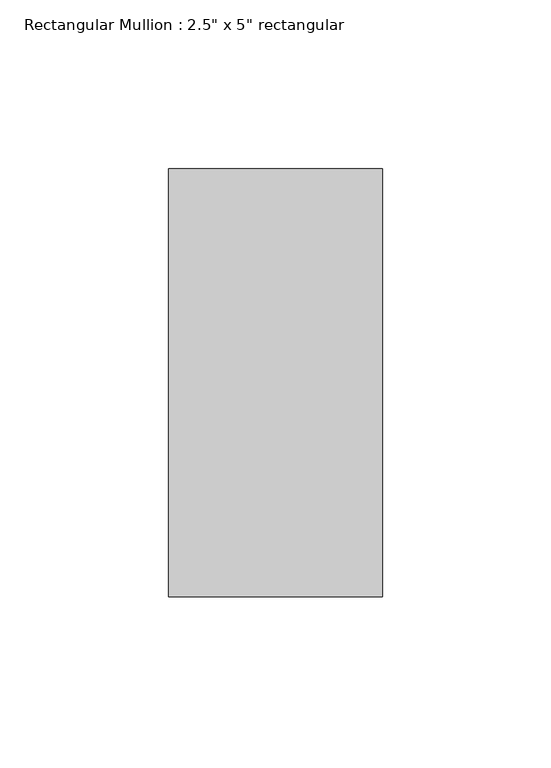
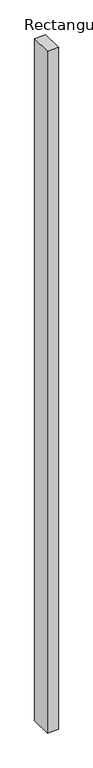
"""IFC4 building model written with IfcOpenShell, lengths in millimetres: member geometry."""

from ifc_helpers import new_model, si_unit, frame, origin, place, context, project, spatial, polyline, outline, extrude, source, transform, mapped, element, save


def member_86c371d5(model_context):
    return source(origin(), model_context, "Body", "SweptSolid", [
        extrude(outline(polyline([(0.0, 63.5), (0.0, -63.5), (-63.5, -63.5), (-63.5, 63.5), (0.0, 63.5)])), frame((0.0, 0.0, -4178.3), z_axis=(0.0, 0.0, 1.0), x_axis=(1.0, 0.0, 0.0)), (0.0, 0.0, 1.0), 4178.3),
    ])


if __name__ == "__main__":
    model = new_model("IFC4")
    model_context = context("Model", 3, world=origin())
    ifc_project = project(units=[si_unit("LENGTHUNIT", "METRE", prefix="MILLI")], contexts=[model_context])
    site = spatial("IfcSite", under=ifc_project)
    building = spatial("IfcBuilding", under=site)
    placement = place(None, origin())
    member_shape = member_86c371d5(model_context)
    element("IfcMember", 1, ObjectType="Rectangular Mullion : 2.5\" x 5\" rectangular", at=placement, inside=building, context=model_context, shape_type="MappedRepresentation", body=[
        mapped(member_shape, transform((0.0, 0.0, 0.0), x_axis=(1.0, 0.0, 0.0), y_axis=(0.0, 1.0, 0.0), z_axis=(0.0, 0.0, 1.0))),
    ])
    save(model, "model.ifc")

# Revit data of these elements
# Type "Rectangular Mullion : 2.5\" x 5\" rectangular"
#   built-in parameter 1007304 = 0.416667 (stored number, unit not read)
#   built-in parameter 1007301 = 0.104167 (stored number, unit not read)
#   built-in parameter 1007300 = 0.104167 (stored number, unit not read)
# Element 1 (IfcMember, "Rectangular Mullion : 2.5\" x 5\" rectangular")
#   Materials on its faces: "Aluminum"
# Materials
#   "Aluminum": class "Metal", colour RGB 247 247 247, transparency 0, Description = "Aluminum 6061", Cost = 0
